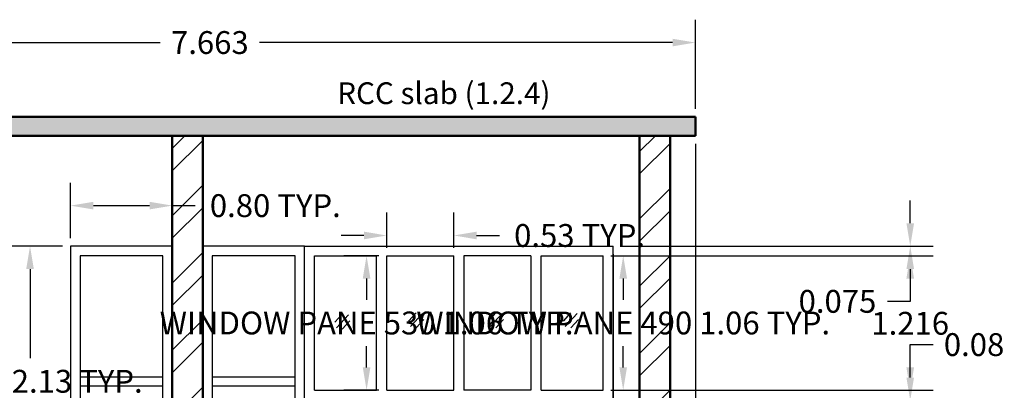
# Model space of a CAD drawing. Units: metres. Extents: x 22.1 to 34.4, y 4.4 to 12.4.
# Tile 8 of 8: x 26.6 to 34.4, y 9.5 to 12.4. Entities that reach past the tile are written whole.
import ezdxf

# ---------------------------------------------------------------- set-up
doc = ezdxf.new("R2010")
doc.units = ezdxf.units.M
doc.header["$MEASUREMENT"] = 0
for name, color, linetype, lineweight in [('A-ANNO-DIMS', 2, 'Continuous', 18), ('A-ANNO-TEXT', 7, 'Continuous', 18), ('A-DOOR', 4, 'Continuous', 25), ('A-GLAZ', 4, 'Continuous', 25), ('A-WALL', 7, 'Continuous', 50), ('A-WALL-PATT', 8, 'Continuous', 18), ('S-SLAB', 1, 'Continuous', 50), ('S-SLAB-PATT', 8, 'Continuous', 13)]:
    doc.layers.add(name, color=color, linetype=linetype, lineweight=lineweight)
doc.styles.get("Standard").update_dxf_attribs({"font": 'arial.ttf'})
doc.dimstyles.get("Standard").update_dxf_attribs({"dimtxt": 0.18, "dimasz": 0.18, "dimexe": 0.18, "dimexo": 0.0625, "dimgap": 0.09, "dimtad": 0, "dimtih": 1, "dimtoh": 1, "dimzin": 0, "dimdsep": 46, "dimtxsty": 'Standard', "dimcen": 0.09, "dimadec": 0, "dimazin": 0, "dimtfac": 1, "dimtofl": 0, "dimtmove": 0, "dimatfit": 3, "dimfxl": 1, "dimtolj": 1, "dimtzin": 0, "dimarcsym": 0})

# ---------------------------------------------------------------- blocks, each defined once
blk = doc.blocks.new('DOOR-800')
for p, q in [((26.4206, 10.6399), (25.6173, 10.6399)), ((25.6173, 10.6399), (25.6173, 8.5099)), ((26.4206, 8.5099), (26.4206, 10.6399)), ((25.6923, 10.5649), (25.6923, 8.5849)), ((26.3456, 10.5649), (25.6923, 10.5649)), ((26.3456, 8.5849), (26.3456, 10.5649)), ((25.6923, 9.6099), (26.3456, 9.6099)), ((25.6923, 9.5399), (26.3456, 9.5399)), ((25.6923, 8.5849), (26.3456, 8.5849)), ((25.6173, 8.5099), (26.4206, 8.5099))]:
    blk.add_line(p, q)
blk = doc.blocks.new('WIN-PANE-490')
for p, q in [((0.0003, 1.0609), (0.4893, 1.0609)), ((0.0003, -0.0001), (0.0003, 1.0609)), ((0.4893, -0.0001), (0.4893, 1.0609)), ((0.0003, -0.0001), (0.4893, -0.0001))]:
    blk.add_line(p, q)
blk = doc.blocks.new('WIN-PANE-530')
for p, q in [((0.0003, -0.0001), (0.0003, 1.0609)), ((0.0003, 1.0609), (0.5293, 1.0609)), ((0.5293, -0.0001), (0.5293, 1.0609)), ((0.0003, -0.0001), (0.5293, -0.0001))]:
    blk.add_line(p, q)
blk = doc.blocks.new('GLASS-MARK')
for p, q in [((29.132, 10.0396), (29.1914, 10.105)), ((29.1465, 9.996), (29.2401, 10.0991)), ((29.1913, 9.9859), (29.2507, 10.0513))]:
    blk.add_line(p, q)
blk = doc.blocks.new('*D16')
at = {"layer": 'A-ANNO-DIMS', "color": 0, "lineweight": -2, "transparency": 16777216}
for p, q in [((26.9843, 10.6399), (26.5473, 10.6399)), ((26.7273, 10.4599), (26.7273, 9.7581)), ((26.7273, 8.6899), (26.7273, 9.3917)), ((26.9843, 8.5099), (26.5473, 8.5099))]:
    blk.add_line(p, q, dxfattribs=at)
at = {"layer": 'A-ANNO-DIMS', "color": 0, "transparency": 16777216}
for points in [[(26.6973, 10.4599), (26.7573, 10.4599), (26.7273, 10.6399)], [(26.6973, 8.6899), (26.7573, 8.6899), (26.7273, 8.5099)]]:
    blk.add_solid(points, dxfattribs=at)
at = {"layer": 'Defpoints', "color": 0, "transparency": 16777216}
for p in [(26.7273, 10.6399), (27.0468, 10.6399), (27.0468, 8.5099)]:
    blk.add_point(p, dxfattribs=at)
at = {"layer": 'A-ANNO-DIMS', "color": 0, "transparency": 16777216, "insert": (26.7273, 9.5749), "char_height": 0.18, "attachment_point": 5}
blk.add_mtext('\\A1;DOOR 2.13 TYP.', dxfattribs=at)
blk = doc.blocks.new('*D17')
at = {"layer": 'A-ANNO-DIMS', "color": 0, "lineweight": -2, "transparency": 16777216}
for p, q in [((27.0468, 10.7024), (27.0468, 11.1394)), ((27.8501, 10.7024), (27.8501, 11.1394)), ((27.2268, 10.9594), (27.6701, 10.9594)), ((27.8501, 10.9594), (28.0301, 10.9594))]:
    blk.add_line(p, q, dxfattribs=at)
at = {"layer": 'A-ANNO-DIMS', "color": 0, "transparency": 16777216}
for points in [[(27.2268, 10.9894), (27.2268, 10.9294), (27.0468, 10.9594)], [(27.6701, 10.9894), (27.6701, 10.9294), (27.8501, 10.9594)]]:
    blk.add_solid(points, dxfattribs=at)
at = {"layer": 'Defpoints', "color": 0, "transparency": 16777216}
for p in [(27.8501, 10.9594), (27.0468, 10.6399), (27.8501, 10.6399)]:
    blk.add_point(p, dxfattribs=at)
at = {"layer": 'A-ANNO-DIMS', "color": 0, "transparency": 16777216, "insert": (28.663, 10.9594), "char_height": 0.18, "attachment_point": 5}
blk.add_mtext('\\A1;0.80 TYP.', dxfattribs=at)
blk = doc.blocks.new('*D18')
at = {"layer": 'A-ANNO-DIMS', "color": 0, "lineweight": -2, "transparency": 16777216}
for p, q in [((31.3118, 10.5649), (31.5885, 10.5649)), ((31.4085, 10.3849), (31.4085, 10.2175)), ((31.4085, 9.6839), (31.4085, 9.8513)), ((31.3118, 9.5039), (31.5885, 9.5039))]:
    blk.add_line(p, q, dxfattribs=at)
at = {"layer": 'A-ANNO-DIMS', "color": 0, "transparency": 16777216}
for points in [[(31.3785, 10.3849), (31.4385, 10.3849), (31.4085, 10.5649)], [(31.3785, 9.6839), (31.4385, 9.6839), (31.4085, 9.5039)]]:
    blk.add_solid(points, dxfattribs=at)
at = {"layer": 'Defpoints', "color": 0, "transparency": 16777216}
for p in [(31.2493, 10.5649), (31.4085, 10.5649), (31.2493, 9.5039)]:
    blk.add_point(p, dxfattribs=at)
at = {"layer": 'A-ANNO-DIMS', "color": 0, "transparency": 16777216, "insert": (31.4085, 10.0344), "char_height": 0.18, "attachment_point": 5}
blk.add_mtext('\\A1;WINDOW PANE 490 1.06 TYP.', dxfattribs=at)
blk = doc.blocks.new('*D19')
at = {"layer": 'A-ANNO-DIMS', "color": 0, "lineweight": -2, "transparency": 16777216}
for p, q in [((30.7603, 9.4414), (30.7603, 9.1648)), ((31.2493, 9.4414), (31.2493, 9.1648)), ((30.5803, 9.3448), (30.4003, 9.3448)), ((31.4293, 9.3448), (31.6093, 9.3448))]:
    blk.add_line(p, q, dxfattribs=at)
at = {"layer": 'A-ANNO-DIMS', "color": 0, "transparency": 16777216}
for points in [[(30.5803, 9.3748), (30.5803, 9.3148), (30.7603, 9.3448)], [(31.4293, 9.3748), (31.4293, 9.3148), (31.2493, 9.3448)]]:
    blk.add_solid(points, dxfattribs=at)
at = {"layer": 'Defpoints', "color": 0, "transparency": 16777216}
for p in [(30.7603, 9.5039), (31.2493, 9.5039), (31.2493, 9.3448)]:
    blk.add_point(p, dxfattribs=at)
at = {"layer": 'A-ANNO-DIMS', "color": 0, "transparency": 16777216, "insert": (32.2423, 9.3448), "char_height": 0.18, "attachment_point": 5}
blk.add_mtext('\\A1;0.49 TYP.', dxfattribs=at)
blk = doc.blocks.new('*D20')
at = {"layer": 'A-ANNO-DIMS', "color": 0, "lineweight": -2, "transparency": 16777216}
for p, q in [((29.4798, 10.5649), (29.2032, 10.5649)), ((29.3832, 10.3849), (29.3832, 10.2176)), ((29.3832, 9.6839), (29.3832, 9.8512)), ((29.4798, 9.5039), (29.2032, 9.5039))]:
    blk.add_line(p, q, dxfattribs=at)
at = {"layer": 'A-ANNO-DIMS', "color": 0, "transparency": 16777216}
for points in [[(29.3532, 10.3849), (29.4132, 10.3849), (29.3832, 10.5649)], [(29.3532, 9.6839), (29.4132, 9.6839), (29.3832, 9.5039)]]:
    blk.add_solid(points, dxfattribs=at)
at = {"layer": 'Defpoints', "color": 0, "transparency": 16777216}
for p in [(29.3832, 10.5649), (29.5423, 10.5649), (29.5423, 9.5039)]:
    blk.add_point(p, dxfattribs=at)
at = {"layer": 'A-ANNO-DIMS', "color": 0, "transparency": 16777216, "insert": (29.3832, 10.0344), "char_height": 0.18, "attachment_point": 5}
blk.add_mtext('\\A1;WINDOW PANE 530 1.06 TYP.', dxfattribs=at)
blk = doc.blocks.new('*D21')
at = {"layer": 'A-ANNO-DIMS', "color": 0, "lineweight": -2, "transparency": 16777216}
for p, q in [((29.5423, 10.6274), (29.5423, 10.9041)), ((30.0713, 10.6274), (30.0713, 10.9041)), ((29.3623, 10.7241), (29.1823, 10.7241)), ((30.2513, 10.7241), (30.4313, 10.7241))]:
    blk.add_line(p, q, dxfattribs=at)
at = {"layer": 'A-ANNO-DIMS', "color": 0, "transparency": 16777216}
for points in [[(29.3623, 10.7541), (29.3623, 10.6941), (29.5423, 10.7241)], [(30.2513, 10.7541), (30.2513, 10.6941), (30.0713, 10.7241)]]:
    blk.add_solid(points, dxfattribs=at)
at = {"layer": 'Defpoints', "color": 0, "transparency": 16777216}
for p in [(30.0713, 10.7241), (29.5423, 10.5649), (30.0713, 10.5649)]:
    blk.add_point(p, dxfattribs=at)
at = {"layer": 'A-ANNO-DIMS', "color": 0, "transparency": 16777216, "insert": (31.0643, 10.7241), "char_height": 0.18, "attachment_point": 5}
blk.add_mtext('\\A1;0.53 TYP.', dxfattribs=at)
blk = doc.blocks.new('*D23')
at = {"layer": 'A-ANNO-DIMS', "color": 0, "lineweight": -2, "transparency": 16777216}
for p, q in [((28.0901, 11.4474), (28.0901, 6.2449)), ((31.5381, 11.4474), (31.5381, 6.2449)), ((28.2701, 6.4249), (29.4202, 6.4249)), ((31.3581, 6.4249), (30.2079, 6.4249))]:
    blk.add_line(p, q, dxfattribs=at)
at = {"layer": 'A-ANNO-DIMS', "color": 0, "transparency": 16777216}
for points in [[(28.2701, 6.4549), (28.2701, 6.3949), (28.0901, 6.4249)], [(31.3581, 6.4549), (31.3581, 6.3949), (31.5381, 6.4249)]]:
    blk.add_solid(points, dxfattribs=at)
at = {"layer": 'Defpoints', "color": 0, "transparency": 16777216}
for p in [(28.0901, 11.5099), (31.5381, 11.5099), (31.5381, 6.4249)]:
    blk.add_point(p, dxfattribs=at)
at = {"layer": 'A-ANNO-DIMS', "color": 0, "transparency": 16777216, "insert": (29.8141, 6.4249), "char_height": 0.18, "attachment_point": 5}
blk.add_mtext('\\A1;3.448', dxfattribs=at)
blk = doc.blocks.new('*D26')
at = {"layer": 'A-ANNO-DIMS', "color": 0, "lineweight": -2, "transparency": 16777216}
for p, q in [((27.8501, 11.4474), (27.8501, 6.2449)), ((28.0901, 11.4474), (28.0901, 6.2449)), ((27.6701, 6.4249), (27.4901, 6.4249)), ((28.2701, 6.4249), (28.4501, 6.4249))]:
    blk.add_line(p, q, dxfattribs=at)
at = {"layer": 'A-ANNO-DIMS', "color": 0, "transparency": 16777216}
for points in [[(27.6701, 6.4549), (27.6701, 6.3949), (27.8501, 6.4249)], [(28.2701, 6.4549), (28.2701, 6.3949), (28.0901, 6.4249)]]:
    blk.add_solid(points, dxfattribs=at)
at = {"layer": 'Defpoints', "color": 0, "transparency": 16777216}
for p in [(27.8501, 11.5099), (28.0901, 11.5099), (28.0901, 6.4249)]:
    blk.add_point(p, dxfattribs=at)
at = {"layer": 'A-ANNO-DIMS', "color": 0, "transparency": 16777216, "insert": (28.7735, 6.4249), "char_height": 0.18, "attachment_point": 5}
blk.add_mtext('\\A1;0.24', dxfattribs=at)
blk = doc.blocks.new('*D27')
at = {"layer": 'A-ANNO-DIMS', "color": 0, "lineweight": -2, "transparency": 16777216}
for p, q in [((31.5381, 11.4474), (31.5381, 6.2449)), ((31.7781, 11.4474), (31.7781, 6.2449)), ((31.3581, 6.4249), (31.1781, 6.4249)), ((31.9581, 6.4249), (32.1381, 6.4249))]:
    blk.add_line(p, q, dxfattribs=at)
at = {"layer": 'A-ANNO-DIMS', "color": 0, "transparency": 16777216}
for points in [[(31.3581, 6.4549), (31.3581, 6.3949), (31.5381, 6.4249)], [(31.9581, 6.4549), (31.9581, 6.3949), (31.7781, 6.4249)]]:
    blk.add_solid(points, dxfattribs=at)
at = {"layer": 'Defpoints', "color": 0, "transparency": 16777216}
for p in [(31.5381, 11.5099), (31.7781, 11.5099), (31.7781, 6.4249)]:
    blk.add_point(p, dxfattribs=at)
at = {"layer": 'A-ANNO-DIMS', "color": 0, "transparency": 16777216, "insert": (32.4615, 6.4249), "char_height": 0.18, "attachment_point": 5}
blk.add_mtext('\\A1;0.24', dxfattribs=at)
blk = doc.blocks.new('*D28')
at = {"layer": 'A-ANNO-DIMS', "color": 0, "lineweight": -2, "transparency": 16777216}
for p, q in [((31.7781, 11.4474), (31.7781, 6.2449)), ((31.9781, 11.4474), (31.9781, 6.2449)), ((31.5981, 6.4249), (31.4181, 6.4249)), ((32.1581, 6.4249), (32.3381, 6.4249))]:
    blk.add_line(p, q, dxfattribs=at)
at = {"layer": 'A-ANNO-DIMS', "color": 0, "transparency": 16777216}
for points in [[(31.5981, 6.4549), (31.5981, 6.3949), (31.7781, 6.4249)], [(32.1581, 6.4549), (32.1581, 6.3949), (31.9781, 6.4249)]]:
    blk.add_solid(points, dxfattribs=at)
at = {"layer": 'Defpoints', "color": 0, "transparency": 16777216}
for p in [(31.7781, 11.5099), (31.9781, 11.5099), (31.9781, 6.4249)]:
    blk.add_point(p, dxfattribs=at)
at = {"layer": 'A-ANNO-DIMS', "color": 0, "transparency": 16777216, "insert": (32.6615, 6.4249), "char_height": 0.18, "attachment_point": 5}
blk.add_mtext('\\A1;0.20', dxfattribs=at)
blk = doc.blocks.new('*D29')
at = {"layer": 'A-ANNO-DIMS', "color": 0, "lineweight": -2, "transparency": 16777216}
for p, q in [((24.3149, 11.7224), (24.3149, 12.4249)), ((31.9781, 11.7224), (31.9781, 12.4249)), ((24.4949, 12.2449), (27.7535, 12.2449)), ((31.7981, 12.2449), (28.5394, 12.2449))]:
    blk.add_line(p, q, dxfattribs=at)
at = {"layer": 'A-ANNO-DIMS', "color": 0, "transparency": 16777216}
for points in [[(24.4949, 12.2749), (24.4949, 12.2149), (24.3149, 12.2449)], [(31.7981, 12.2749), (31.7981, 12.2149), (31.9781, 12.2449)]]:
    blk.add_solid(points, dxfattribs=at)
at = {"layer": 'Defpoints', "color": 0, "transparency": 16777216}
for p in [(31.9781, 12.2449), (24.3149, 11.6599), (31.9781, 11.6599)]:
    blk.add_point(p, dxfattribs=at)
at = {"layer": 'A-ANNO-DIMS', "color": 0, "transparency": 16777216, "insert": (28.1465, 12.2449), "char_height": 0.18, "attachment_point": 5}
blk.add_mtext('\\A1;7.663', dxfattribs=at)
blk = doc.blocks.new('*D33')
at = {"layer": 'A-ANNO-DIMS', "color": 0, "lineweight": -2, "transparency": 16777216}
for p, q in [((31.5381, 11.4474), (31.5381, 6.2449)), ((31.3293, 10.5774), (31.3293, 6.2449)), ((31.1493, 6.4249), (30.9693, 6.4249)), ((31.7181, 6.4249), (31.8981, 6.4249))]:
    blk.add_line(p, q, dxfattribs=at)
at = {"layer": 'A-ANNO-DIMS', "color": 0, "transparency": 16777216}
for points in [[(31.1493, 6.4549), (31.1493, 6.3949), (31.3293, 6.4249)], [(31.7181, 6.4549), (31.7181, 6.3949), (31.5381, 6.4249)]]:
    blk.add_solid(points, dxfattribs=at)
at = {"layer": 'Defpoints', "color": 0, "transparency": 16777216}
for p in [(31.5381, 11.5099), (31.3293, 10.6399), (31.5381, 6.4249)]:
    blk.add_point(p, dxfattribs=at)
at = {"layer": 'A-ANNO-DIMS', "color": 0, "transparency": 16777216, "insert": (32.2045, 6.4249), "char_height": 0.18, "attachment_point": 5}
blk.add_mtext('\\A1;0.21', dxfattribs=at)
blk = doc.blocks.new('*D40')
at = {"layer": 'A-ANNO-DIMS', "color": 0, "lineweight": -2, "transparency": 16777216}
for p, q in [((31.3918, 10.6399), (33.8537, 10.6399)), ((33.6737, 10.4599), (33.6737, 10.2138)), ((33.6737, 9.6039), (33.6737, 9.85)), ((31.3918, 9.4239), (33.8537, 9.4239))]:
    blk.add_line(p, q, dxfattribs=at)
at = {"layer": 'A-ANNO-DIMS', "color": 0, "transparency": 16777216}
for points in [[(33.6437, 10.4599), (33.7037, 10.4599), (33.6737, 10.6399)], [(33.6437, 9.6039), (33.7037, 9.6039), (33.6737, 9.4239)]]:
    blk.add_solid(points, dxfattribs=at)
at = {"layer": 'Defpoints', "color": 0, "transparency": 16777216}
for p in [(31.3293, 10.6399), (31.3293, 9.4239), (33.6737, 9.4239)]:
    blk.add_point(p, dxfattribs=at)
at = {"layer": 'A-ANNO-DIMS', "color": 0, "transparency": 16777216, "insert": (33.6737, 10.0319), "char_height": 0.18, "attachment_point": 5}
blk.add_mtext('\\A1;1.216', dxfattribs=at)
blk = doc.blocks.new('*D41')
at = {"layer": 'A-ANNO-DIMS', "color": 0, "lineweight": -2, "transparency": 16777216}
for p, q in [((33.6737, 10.8199), (33.6737, 10.9999)), ((31.3918, 10.6399), (33.8537, 10.6399)), ((31.3118, 10.5649), (33.8537, 10.5649)), ((33.6737, 10.3849), (33.6737, 10.2049)), ((33.6737, 10.2049), (33.4937, 10.2049))]:
    blk.add_line(p, q, dxfattribs=at)
at = {"layer": 'A-ANNO-DIMS', "color": 0, "transparency": 16777216}
for points in [[(33.6437, 10.8199), (33.7037, 10.8199), (33.6737, 10.6399)], [(33.6437, 10.3849), (33.7037, 10.3849), (33.6737, 10.5649)]]:
    blk.add_solid(points, dxfattribs=at)
at = {"layer": 'Defpoints', "color": 0, "transparency": 16777216}
for p in [(31.3293, 10.6399), (31.2493, 10.5649), (33.6737, 10.5649)]:
    blk.add_point(p, dxfattribs=at)
at = {"layer": 'A-ANNO-DIMS', "color": 0, "transparency": 16777216, "insert": (33.0993, 10.2049), "char_height": 0.18, "attachment_point": 5}
blk.add_mtext('\\A1;0.075', dxfattribs=at)
blk = doc.blocks.new('*D42')
at = {"layer": 'A-ANNO-DIMS', "color": 0, "lineweight": -2, "transparency": 16777216}
for p, q in [((33.6737, 9.6839), (33.6737, 9.8639)), ((33.6737, 9.8639), (33.8537, 9.8639)), ((31.3118, 9.5039), (33.8537, 9.5039)), ((31.3918, 9.4239), (33.8537, 9.4239)), ((33.6737, 9.2439), (33.6737, 9.0639))]:
    blk.add_line(p, q, dxfattribs=at)
at = {"layer": 'A-ANNO-DIMS', "color": 0, "transparency": 16777216}
for points in [[(33.6437, 9.6839), (33.7037, 9.6839), (33.6737, 9.5039)], [(33.6437, 9.2439), (33.7037, 9.2439), (33.6737, 9.4239)]]:
    blk.add_solid(points, dxfattribs=at)
at = {"layer": 'Defpoints', "color": 0, "transparency": 16777216}
for p in [(31.2493, 9.5039), (33.6737, 9.5039), (31.3293, 9.4239)]:
    blk.add_point(p, dxfattribs=at)
at = {"layer": 'A-ANNO-DIMS', "color": 0, "transparency": 16777216, "insert": (34.1776, 9.8639), "char_height": 0.18, "attachment_point": 5}
blk.add_mtext('\\A1;0.08', dxfattribs=at)

msp = doc.modelspace()

# ---------------------------------------------------------------- hatches: boundary and pattern name
at = {"layer": 'A-WALL-PATT'}
h = msp.add_hatch(dxfattribs=at)
h.set_pattern_fill('ANSI32', color=256)
h.paths.add_polyline_path([(24.7549, 11.5099), (24.5149, 11.5099), (24.5149, 11.1399), (24.7549, 11.1399)])
h.paths.add_polyline_path([(24.7549, 10.6399), (24.5149, 10.6399), (24.5149, 8.5099), (24.6349, 8.5099), (24.7549, 8.5099)])
h.paths.add_polyline_path([(26.5706, 11.5099), (26.4206, 11.5099), (26.4206, 8.5099), (26.5706, 8.5099)])
h.paths.add_polyline_path([(28.0901, 10.6399), (28.0901, 11.5099), (27.8501, 11.5099), (27.8501, 8.5099), (28.0901, 8.5099)])
h.paths.add_polyline_path([(31.7781, 11.5099), (31.5381, 11.5099), (31.5381, 8.5099), (31.6581, 8.5099), (31.7781, 8.5099)])
at = {"layer": 'S-SLAB-PATT'}
h = msp.add_hatch(dxfattribs=at)
h.set_pattern_fill('AR-CONC', color=256, scale=0.04)
h.set_pattern_definition([(50, (0, 0), (0.286904, -0.0251009), [0.03, -0.33]), (355, (0, 0), (-0.0555005, 0.3008769), [0.024, -0.264]), (100.4514, (0.0239, -0.0021), (0.2314035, 0.275776), [0.025496, -0.2804568]), (46.1842, (0, 0.08), (0.4268965, -0.0662077), [0.045, -0.495]), (96.6356, (0.03557, 0.0745), (0.373865, 0.3896474), [0.038244, -0.4206855]), (351.1842, (0, 0.08), (0.373865, 0.3896474), [0.036, -0.396]), (21, (0.04, 0.06), (0.2387628, -0.1610476), [0.03, -0.33]), (326, (0.04, 0.06), (0.0973261, 0.29006), [0.024, -0.264]), (71.4514, (0.0599, 0.04658), (0.336089, 0.1290125), [0.025496, -0.2804568]), (37.5, (0, 0), (0.00486394, 0.13315754), [0, -0.2608, 0, -0.268, 0, -0.265]), (7.5, (0, 0), (0.1052278, 0.1577647), [0, -0.1528, 0, -0.2548, 0, -0.101]), (327.5, (-0.0892, 0), (0.21352897, -0.00902195), [0, -0.1, 0, -0.312, 0, -0.414]), (317.5, (-0.1292, 0), (0.2332745, 0.040042), [0, -0.13, 0, -0.2072, 0, -0.294])])
h.paths.add_polyline_path([(31.9781, 11.6599), (24.3149, 11.6599), (24.3149, 11.5099), (24.5149, 11.5099), (31.7781, 11.5099), (31.9781, 11.5099)])
h.paths.add_polyline_path([(25.1849, 7.2099), (24.9849, 7.2099), (24.0849, 7.2099), (24.0849, 7.0099), (25.1849, 7.0099)])
h.paths.add_polyline_path([(32.2081, 7.2099), (32.0081, 7.2099), (31.1081, 7.2099), (31.1081, 7.0099), (32.2081, 7.0099)])
h.paths.add_polyline_path([(28.5201, 7.2099), (28.3201, 7.2099), (27.4201, 7.2099), (27.4201, 7.0099), (28.5201, 7.0099)])
h.paths.add_polyline_path([(24.7849, 8.5099), (24.6349, 8.5099), (24.5149, 8.5099), (24.4849, 8.5099), (24.4849, 8.4099), (24.7849, 8.4099)])
h.paths.add_polyline_path([(26.6456, 8.5099), (26.3456, 8.5099), (26.3456, 8.4099), (26.6456, 8.4099)])
h.paths.add_polyline_path([(28.1201, 8.5099), (28.0901, 8.5099), (27.8201, 8.5099), (27.8201, 8.4099), (28.1201, 8.4099)])
h.paths.add_polyline_path([(31.8081, 8.5099), (31.6581, 8.5099), (31.5381, 8.5099), (31.5081, 8.5099), (31.5081, 8.4099), (31.8081, 8.4099)])
h.paths.add_polyline_path([(26.3456, 8.3119), (24.7849, 8.3119), (24.7849, 8.1578), (26.3456, 8.1578)])
h.paths.add_polyline_path([(27.8201, 8.3119), (26.6456, 8.3119), (26.6456, 8.1578), (27.8201, 8.1578)])
h.paths.add_polyline_path([(31.5081, 8.3119), (28.1201, 8.3119), (28.1201, 8.1578), (31.5081, 8.1578)])

# ---------------------------------------------------------------- linework, layer by layer
at = {"layer": 'A-GLAZ'}
for p in [(28.8933, 10.6399), (31.3293, 9.4239)]:
    msp.add_line(p, (31.3293, 10.6399), dxfattribs=at)
at = {"layer": 'A-WALL'}
for p, q in [((27.8501, 8.5099), (27.8501, 11.5099)), ((27.8501, 11.5099), (27.9701, 11.5099)), ((28.0901, 11.5099), (27.9701, 11.5099)), ((28.0901, 8.5099), (28.0901, 11.5099)), ((31.5381, 8.5099), (31.5381, 11.5099)), ((31.5381, 11.5099), (31.6581, 11.5099)), ((31.7781, 11.5099), (31.6581, 11.5099)), ((31.7781, 8.5099), (31.7781, 11.5099))]:
    msp.add_line(p, q, dxfattribs=at)
at = {"layer": 'S-SLAB'}
for p, q in [((31.9781, 11.6599), (24.3149, 11.6599)), ((31.9781, 11.5099), (31.9781, 11.6599)), ((24.5149, 11.5099), (31.7781, 11.5099)), ((31.7781, 11.5099), (31.9781, 11.5099))]:
    msp.add_line(p, q, dxfattribs=at)

# ---------------------------------------------------------------- block references
at = {"layer": 'A-DOOR'}
for p in [(1.4295, 0), (2.4728, 0)]:
    msp.add_blockref('DOOR-800', p, dxfattribs=at)
at = {"layer": 'A-GLAZ'}
for name, p in [('WIN-PANE-490', (28.973, 9.504)), ('WIN-PANE-530', (29.542, 9.504)), ('WIN-PANE-490', (30.76, 9.504)), ('GLASS-MARK', (0, 0)), ('GLASS-MARK', (0.5832, 0.0098)), ('GLASS-MARK', (1.213, 0.0098)), ('GLASS-MARK', (1.8042, 0.0098))]:
    msp.add_blockref(name, p, dxfattribs=at)
at = {"layer": 'A-GLAZ', "rotation": 180}
msp.add_blockref('WIN-PANE-530', (30.6807, 10.5648), dxfattribs=at)

# ---------------------------------------------------------------- texts
at = {"layer": 'A-ANNO-TEXT'}
msp.add_text('RCC slab (1.2.4)', height=0.171602, dxfattribs=at).set_placement((29.1515, 11.7597))

# ---------------------------------------------------------------- dimensions: what is measured, and where the dimension line sits
at = {"layer": 'A-ANNO-DIMS'}
for base, p1, p2, override, picture, middle in [((31.9781, 12.2449), (24.3149, 11.6599), (31.9781, 11.6599), {"dimdec": 3, "dimlfac": 1, "dimrnd": 0, "dimzin": 0, "dimdsep": 46, "dimlunit": 2}, '*D29', (28.1465, 12.2449)), ((28.0901, 6.4249), (27.8501, 11.5099), (28.0901, 11.5099), {"dimdec": 2, "dimlfac": 1, "dimrnd": 0, "dimzin": 0, "dimdsep": 46, "dimlunit": 2}, '*D26', (28.7735, 6.4249)), ((31.5381, 6.4249), (28.0901, 11.5099), (31.5381, 11.5099), {"dimdec": 3, "dimlfac": 1, "dimrnd": 0, "dimzin": 0, "dimdsep": 46, "dimlunit": 2}, '*D23', (29.8141, 6.4249)), ((31.5381, 6.4249), (31.3293, 10.6399), (31.5381, 11.5099), {"dimdec": 2, "dimlfac": 1, "dimrnd": 0, "dimzin": 0, "dimdsep": 46, "dimlunit": 2}, '*D33', (32.2045, 6.4249)), ((31.7781, 6.4249), (31.5381, 11.5099), (31.7781, 11.5099), {"dimdec": 2, "dimlfac": 1, "dimrnd": 0, "dimzin": 0, "dimdsep": 46, "dimlunit": 2}, '*D27', (32.4615, 6.4249)), ((31.9781, 6.4249), (31.7781, 11.5099), (31.9781, 11.5099), {"dimdec": 2, "dimlfac": 1, "dimrnd": 0, "dimzin": 0, "dimdsep": 46, "dimlunit": 2}, '*D28', (32.6615, 6.4249))]:
    dim = msp.add_linear_dim(base=base, p1=p1, p2=p2, dimstyle='Standard', override=override, dxfattribs=at)
    dim.commit()
    dim.dimension.update_dxf_attribs({"geometry": picture, "text_midpoint": middle})
for base, p1, p2, picture, middle in [((27.8501, 10.9594), (27.0468, 10.6399), (27.8501, 10.6399), '*D17', (28.663, 10.9594)), ((30.0713, 10.7241), (29.5423, 10.5649), (30.0713, 10.5649), '*D21', (31.0643, 10.7241)), ((31.2493, 9.3448), (30.7603, 9.5039), (31.2493, 9.5039), '*D19', (32.2423, 9.3448))]:
    dim = msp.add_linear_dim(base=base, p1=p1, p2=p2, text='<> TYP.', dimstyle='Standard', override={"dimdec": 2, "dimrnd": 0, "dimzin": 0, "dimlunit": 2}, dxfattribs=at)
    dim.commit()
    dim.dimension.update_dxf_attribs({"geometry": picture, "text_midpoint": middle})
for base, p1, p2, override, picture, middle in [((33.6737, 10.5649), (31.3293, 10.6399), (31.2493, 10.5649), {"dimdec": 3, "dimlfac": 1, "dimrnd": 0, "dimzin": 0, "dimdsep": 46, "dimlunit": 2}, '*D41', (33.0993, 10.2049)), ((33.6737, 9.4239), (31.3293, 10.6399), (31.3293, 9.4239), {"dimdec": 3, "dimlfac": 1, "dimrnd": 0, "dimzin": 0, "dimdsep": 46, "dimlunit": 2}, '*D40', (33.6737, 10.0319)), ((33.6737, 9.5039), (31.3293, 9.4239), (31.2493, 9.5039), {"dimdec": 2, "dimlfac": 1, "dimrnd": 0, "dimzin": 0, "dimdsep": 46, "dimlunit": 2}, '*D42', (34.1776, 9.8639))]:
    dim = msp.add_linear_dim(base=base, p1=p1, p2=p2, angle=90, dimstyle='Standard', override=override, dxfattribs=at)
    dim.commit()
    dim.dimension.update_dxf_attribs({"geometry": picture, "text_midpoint": middle})
for base, p1, p2, text, picture, middle in [((29.3832, 10.5649), (29.5423, 9.5039), (29.5423, 10.5649), 'WINDOW PANE 530 <> TYP.', '*D20', (29.3832, 10.0344)), ((31.4085, 10.5649), (31.2493, 9.5039), (31.2493, 10.5649), 'WINDOW PANE 490 <> TYP.', '*D18', (31.4085, 10.0344)), ((26.7273, 10.6399), (27.0468, 8.5099), (27.0468, 10.6399), 'DOOR <> TYP.', '*D16', (26.7273, 9.5749))]:
    dim = msp.add_linear_dim(base=base, p1=p1, p2=p2, angle=90, text=text, dimstyle='Standard', override={"dimdec": 2, "dimrnd": 0, "dimzin": 0, "dimlunit": 2}, dxfattribs=at)
    dim.commit()
    dim.dimension.update_dxf_attribs({"geometry": picture, "text_midpoint": middle})

doc.saveas('drawing.dxf')
